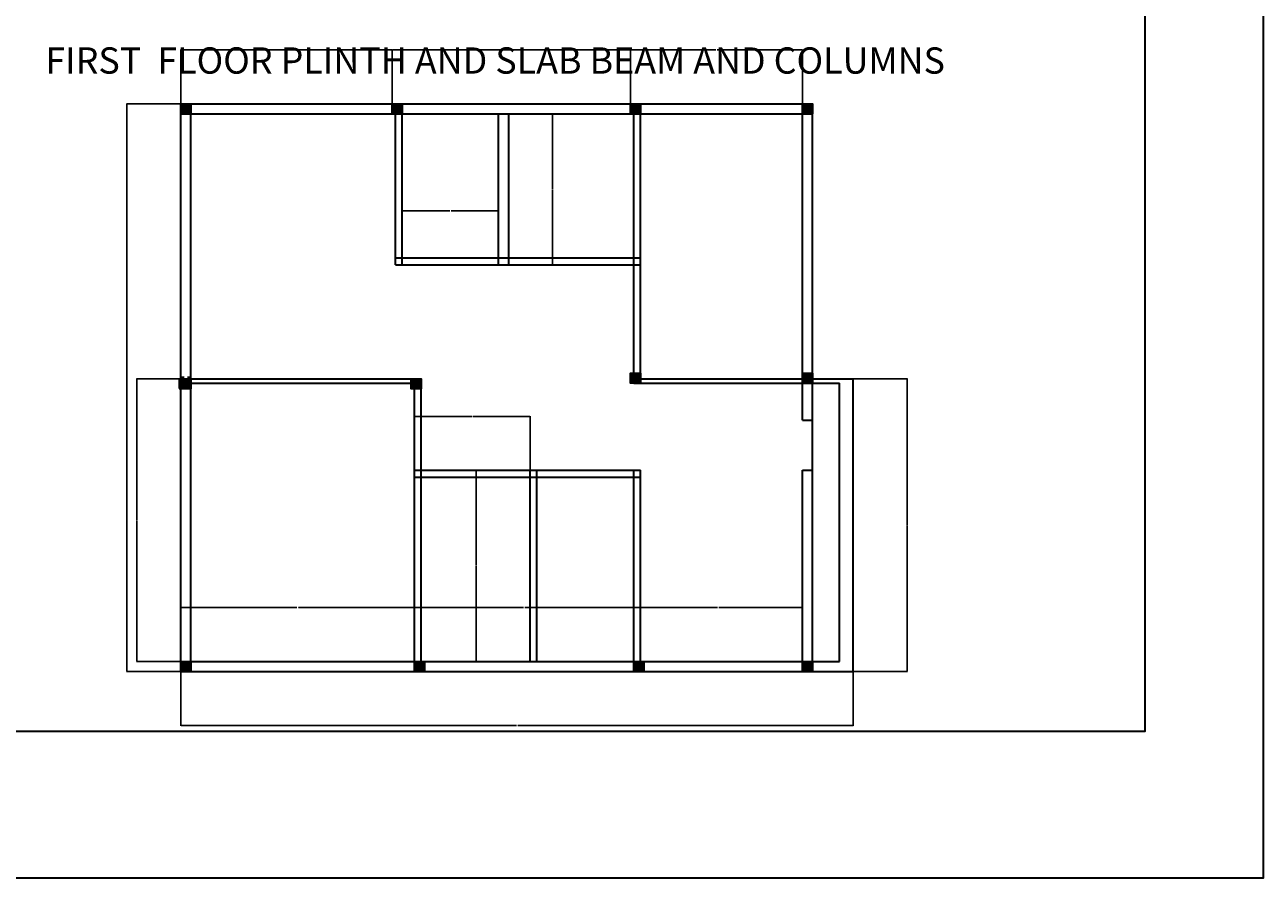
# Model space of a CAD drawing. Units: inches. Extents: x 2286 to 3750, y 1240 to 2345.
# Tile 6 of 7: x 2949 to 3750, y 1240 to 1793. Entities that reach past the tile are written whole.
import ezdxf

# ---------------------------------------------------------------- set-up
doc = ezdxf.new("R2010")
doc.units = ezdxf.units.IN
for name, color, linetype, lineweight in [('A-ANNO-DIMS', 2, 'Continuous', 18), ('A-ANNO-TEXT', 7, 'Continuous', 35), ('A-WALL', 7, 'Continuous', 35), ('S-BEAM', 7, 'Continuous', 30), ('S-COLS', 1, 'Continuous', 35)]:
    doc.layers.add(name, color=color, linetype=linetype, lineweight=lineweight)
doc.styles.get("Standard").update_dxf_attribs({"font": 'arial.ttf'})
doc.dimstyles.get("Standard").update_dxf_attribs({"dimtxt": 0.18, "dimasz": 0.18, "dimexe": 0.18, "dimexo": 0.0625, "dimgap": 0.09, "dimtad": 0, "dimtih": 1, "dimtoh": 1, "dimdec": 4, "dimzin": 0, "dimdsep": 46, "dimtxsty": 'Standard', "dimcen": 0.09, "dimadec": 0, "dimazin": 0, "dimtfac": 1, "dimtdec": 4, "dimtofl": 0, "dimtmove": 0, "dimatfit": 3, "dimfxl": 1, "dimtolj": 1, "dimtzin": 0, "dimarcsym": 0})

# ---------------------------------------------------------------- blocks, each defined once
blk = doc.blocks.new('COL-6p5-SQ')
h = blk.add_hatch(color=256)
h.dxf.hatch_style = 1
h.paths.add_polyline_path([(6.5, 0), (6.5, 6.5), (0, 6.5), (0, 0)])
blk.add_lwpolyline([(0, 6.5), (6.5, 6.5), (6.5, 0), (0, 0)], close=True)
blk = doc.blocks.new('*D20')
at = {"layer": 'A-ANNO-DIMS', "color": 0, "lineweight": -2, "transparency": 16777216}
for p, q in [((3050.31, 1563.7), (3050.31, 1564.79)), ((3050.49, 1564.61), (3052.53, 1564.61)), ((3056.63, 1564.61), (3054.6, 1564.61)), ((3056.81, 1563.7), (3056.81, 1564.79))]:
    blk.add_line(p, q, dxfattribs=at)
at = {"layer": 'A-ANNO-DIMS', "color": 0, "transparency": 16777216}
for points in [[(3050.49, 1564.64), (3050.49, 1564.58), (3050.31, 1564.61)], [(3056.63, 1564.64), (3056.63, 1564.58), (3056.81, 1564.61)]]:
    blk.add_solid(points, dxfattribs=at)
at = {"layer": 'Defpoints', "color": 0, "transparency": 16777216}
for p in [(3050.31, 1564.61), (3050.31, 1563.64), (3056.81, 1563.64)]:
    blk.add_point(p, dxfattribs=at)
at = {"layer": 'A-ANNO-DIMS', "color": 0, "transparency": 16777216, "insert": (3053.56, 1564.61), "char_height": 0.18, "attachment_point": 5}
blk.add_mtext('\\A1;COLUMN 7 TYP.', dxfattribs=at)
blk = doc.blocks.new('*D21')
at = {"layer": 'A-ANNO-DIMS', "color": 0, "lineweight": -2, "transparency": 16777216}
for p, q in [((3050.25, 1563.64), (3049.16, 1563.64)), ((3049.34, 1563.46), (3049.34, 1560.57)), ((3050.25, 1557.14), (3049.16, 1557.14)), ((3049.34, 1557.32), (3049.34, 1560.21))]:
    blk.add_line(p, q, dxfattribs=at)
at = {"layer": 'A-ANNO-DIMS', "color": 0, "transparency": 16777216}
for points in [[(3049.31, 1563.46), (3049.37, 1563.46), (3049.34, 1563.64)], [(3049.31, 1557.32), (3049.37, 1557.32), (3049.34, 1557.14)]]:
    blk.add_solid(points, dxfattribs=at)
at = {"layer": 'Defpoints', "color": 0, "transparency": 16777216}
for p in [(3050.31, 1563.64), (3049.34, 1557.14), (3050.31, 1557.14)]:
    blk.add_point(p, dxfattribs=at)
at = {"layer": 'A-ANNO-DIMS', "color": 0, "transparency": 16777216, "insert": (3049.34, 1560.39), "char_height": 0.18, "attachment_point": 5}
blk.add_mtext('\\A1;7 TYP.', dxfattribs=at)
blk = doc.blocks.new('*D109')
at = {"layer": 'A-ANNO-DIMS', "color": 0, "lineweight": -2, "transparency": 16777216}
for p, q in [((3050.31, 1374.12), (3050.31, 1339.1)), ((3485.18, 1374.12), (3485.18, 1339.1)), ((3050.49, 1339.28), (3267.35, 1339.28)), ((3485, 1339.28), (3268.14, 1339.28))]:
    blk.add_line(p, q, dxfattribs=at)
at = {"layer": 'A-ANNO-DIMS', "color": 0, "transparency": 16777216}
for points in [[(3050.49, 1339.31), (3050.49, 1339.25), (3050.31, 1339.28)], [(3485, 1339.31), (3485, 1339.25), (3485.18, 1339.28)]]:
    blk.add_solid(points, dxfattribs=at)
at = {"layer": 'Defpoints', "color": 0, "transparency": 16777216}
for p in [(3050.31, 1374.18), (3485.18, 1374.18), (3485.18, 1339.28)]:
    blk.add_point(p, dxfattribs=at)
at = {"layer": 'A-ANNO-DIMS', "color": 0, "transparency": 16777216, "insert": (3267.74, 1339.28), "char_height": 0.18, "attachment_point": 5}
blk.add_mtext('\\A1;434.9', dxfattribs=at)
blk = doc.blocks.new('*D110')
at = {"layer": 'A-ANNO-DIMS', "color": 0, "lineweight": -2, "transparency": 16777216}
for p, q in [((3050.25, 1741.52), (3015.23, 1741.52)), ((3015.41, 1741.34), (3015.41, 1558.03)), ((3015.41, 1374.36), (3015.41, 1557.67)), ((3050.24, 1374.18), (3015.23, 1374.18))]:
    blk.add_line(p, q, dxfattribs=at)
at = {"layer": 'A-ANNO-DIMS', "color": 0, "transparency": 16777216}
for points in [[(3015.38, 1741.34), (3015.44, 1741.34), (3015.41, 1741.52)], [(3015.38, 1374.36), (3015.44, 1374.36), (3015.41, 1374.18)]]:
    blk.add_solid(points, dxfattribs=at)
at = {"layer": 'Defpoints', "color": 0, "transparency": 16777216}
for p in [(3015.41, 1741.52), (3050.31, 1741.52), (3050.31, 1374.18)]:
    blk.add_point(p, dxfattribs=at)
at = {"layer": 'A-ANNO-DIMS', "color": 0, "transparency": 16777216, "insert": (3015.41, 1557.85), "char_height": 0.18, "attachment_point": 5}
blk.add_mtext('\\A1;367.34', dxfattribs=at)
blk = doc.blocks.new('*D111')
at = {"layer": 'A-ANNO-DIMS', "color": 0, "lineweight": -2, "transparency": 16777216}
for p, q in [((3050.31, 1741.58), (3050.31, 1776.61)), ((3050.49, 1776.43), (3118.19, 1776.43)), ((3186.8, 1776.43), (3119.1, 1776.43)), ((3186.98, 1741.58), (3186.98, 1776.61))]:
    blk.add_line(p, q, dxfattribs=at)
at = {"layer": 'A-ANNO-DIMS', "color": 0, "transparency": 16777216}
for points in [[(3050.49, 1776.46), (3050.49, 1776.4), (3050.31, 1776.43)], [(3186.8, 1776.46), (3186.8, 1776.4), (3186.98, 1776.43)]]:
    blk.add_solid(points, dxfattribs=at)
at = {"layer": 'Defpoints', "color": 0, "transparency": 16777216}
for p in [(3186.98, 1776.43), (3050.31, 1741.52), (3186.98, 1741.52)]:
    blk.add_point(p, dxfattribs=at)
at = {"layer": 'A-ANNO-DIMS', "color": 0, "transparency": 16777216, "insert": (3118.65, 1776.43), "char_height": 0.18, "attachment_point": 5}
blk.add_mtext('\\A1;136.67', dxfattribs=at)
blk = doc.blocks.new('*D112')
at = {"layer": 'A-ANNO-DIMS', "color": 0, "lineweight": -2, "transparency": 16777216}
for p, q in [((3186.98, 1741.58), (3186.98, 1776.61)), ((3187.16, 1776.43), (3263.54, 1776.43)), ((3340.83, 1776.43), (3264.45, 1776.43)), ((3341.01, 1741.58), (3341.01, 1776.61))]:
    blk.add_line(p, q, dxfattribs=at)
at = {"layer": 'A-ANNO-DIMS', "color": 0, "transparency": 16777216}
for points in [[(3187.16, 1776.46), (3187.16, 1776.4), (3186.98, 1776.43)], [(3340.83, 1776.46), (3340.83, 1776.4), (3341.01, 1776.43)]]:
    blk.add_solid(points, dxfattribs=at)
at = {"layer": 'Defpoints', "color": 0, "transparency": 16777216}
for p in [(3341.01, 1776.43), (3186.98, 1741.52), (3341.01, 1741.52)]:
    blk.add_point(p, dxfattribs=at)
at = {"layer": 'A-ANNO-DIMS', "color": 0, "transparency": 16777216, "insert": (3264, 1776.43), "char_height": 0.18, "attachment_point": 5}
blk.add_mtext('\\A1;154.03', dxfattribs=at)
blk = doc.blocks.new('*D113')
at = {"layer": 'A-ANNO-DIMS', "color": 0, "lineweight": -2, "transparency": 16777216}
for p, q in [((3341.01, 1741.58), (3341.01, 1776.61)), ((3341.19, 1776.43), (3396.23, 1776.43)), ((3452.19, 1776.43), (3397.14, 1776.43)), ((3452.37, 1741.58), (3452.37, 1776.61))]:
    blk.add_line(p, q, dxfattribs=at)
at = {"layer": 'A-ANNO-DIMS', "color": 0, "transparency": 16777216}
for points in [[(3341.19, 1776.46), (3341.19, 1776.4), (3341.01, 1776.43)], [(3452.19, 1776.46), (3452.19, 1776.4), (3452.37, 1776.43)]]:
    blk.add_solid(points, dxfattribs=at)
at = {"layer": 'Defpoints', "color": 0, "transparency": 16777216}
for p in [(3452.37, 1776.43), (3341.01, 1741.52), (3452.37, 1741.52)]:
    blk.add_point(p, dxfattribs=at)
at = {"layer": 'A-ANNO-DIMS', "color": 0, "transparency": 16777216, "insert": (3396.69, 1776.43), "char_height": 0.18, "attachment_point": 5}
blk.add_mtext('\\A1;111.36', dxfattribs=at)
blk = doc.blocks.new('*D114')
at = {"layer": 'A-ANNO-DIMS', "color": 0, "lineweight": -2, "transparency": 16777216}
for p, q in [((3050.31, 1380.74), (3050.31, 1415.76)), ((3050.49, 1415.58), (3125.42, 1415.58)), ((3201.26, 1415.58), (3126.33, 1415.58)), ((3201.44, 1380.74), (3201.44, 1415.76))]:
    blk.add_line(p, q, dxfattribs=at)
at = {"layer": 'A-ANNO-DIMS', "color": 0, "transparency": 16777216}
for points in [[(3050.49, 1415.61), (3050.49, 1415.55), (3050.31, 1415.58)], [(3201.26, 1415.61), (3201.26, 1415.55), (3201.44, 1415.58)]]:
    blk.add_solid(points, dxfattribs=at)
at = {"layer": 'Defpoints', "color": 0, "transparency": 16777216}
for p in [(3201.44, 1415.58), (3050.31, 1380.68), (3201.44, 1380.68)]:
    blk.add_point(p, dxfattribs=at)
at = {"layer": 'A-ANNO-DIMS', "color": 0, "transparency": 16777216, "insert": (3125.87, 1415.58), "char_height": 0.18, "attachment_point": 5}
blk.add_mtext('\\A1;151.13', dxfattribs=at)
blk = doc.blocks.new('*D115')
at = {"layer": 'A-ANNO-DIMS', "color": 0, "lineweight": -2, "transparency": 16777216}
for p, q in [((3201.44, 1380.74), (3201.44, 1415.76)), ((3201.62, 1415.58), (3271.85, 1415.58)), ((3342.99, 1415.58), (3272.76, 1415.58)), ((3343.17, 1380.74), (3343.17, 1415.76))]:
    blk.add_line(p, q, dxfattribs=at)
at = {"layer": 'A-ANNO-DIMS', "color": 0, "transparency": 16777216}
for points in [[(3201.62, 1415.61), (3201.62, 1415.55), (3201.44, 1415.58)], [(3342.99, 1415.61), (3342.99, 1415.55), (3343.17, 1415.58)]]:
    blk.add_solid(points, dxfattribs=at)
at = {"layer": 'Defpoints', "color": 0, "transparency": 16777216}
for p in [(3343.17, 1415.58), (3201.44, 1380.68), (3343.17, 1380.68)]:
    blk.add_point(p, dxfattribs=at)
at = {"layer": 'A-ANNO-DIMS', "color": 0, "transparency": 16777216, "insert": (3272.3, 1415.58), "char_height": 0.18, "attachment_point": 5}
blk.add_mtext('\\A1;141.73', dxfattribs=at)
blk = doc.blocks.new('*D116')
at = {"layer": 'A-ANNO-DIMS', "color": 0, "lineweight": -2, "transparency": 16777216}
for p, q in [((3343.17, 1380.74), (3343.17, 1415.76)), ((3343.35, 1415.58), (3397.39, 1415.58)), ((3452.19, 1415.58), (3398.15, 1415.58)), ((3452.37, 1380.74), (3452.37, 1415.76))]:
    blk.add_line(p, q, dxfattribs=at)
at = {"layer": 'A-ANNO-DIMS', "color": 0, "transparency": 16777216}
for points in [[(3343.35, 1415.61), (3343.35, 1415.55), (3343.17, 1415.58)], [(3452.19, 1415.61), (3452.19, 1415.55), (3452.37, 1415.58)]]:
    blk.add_solid(points, dxfattribs=at)
at = {"layer": 'Defpoints', "color": 0, "transparency": 16777216}
for p in [(3452.37, 1415.58), (3343.17, 1380.68), (3452.37, 1380.68)]:
    blk.add_point(p, dxfattribs=at)
at = {"layer": 'A-ANNO-DIMS', "color": 0, "transparency": 16777216, "insert": (3397.77, 1415.58), "char_height": 0.18, "attachment_point": 5}
blk.add_mtext('\\A1;109.2', dxfattribs=at)
blk = doc.blocks.new('*D117')
at = {"layer": 'A-ANNO-DIMS', "color": 0, "lineweight": -2, "transparency": 16777216}
for p, q in [((3056.75, 1563.64), (3021.73, 1563.64)), ((3021.91, 1563.46), (3021.91, 1472.34)), ((3021.91, 1380.86), (3021.91, 1471.98)), ((3056.74, 1380.68), (3021.73, 1380.68))]:
    blk.add_line(p, q, dxfattribs=at)
at = {"layer": 'A-ANNO-DIMS', "color": 0, "transparency": 16777216}
for points in [[(3021.88, 1563.46), (3021.94, 1563.46), (3021.91, 1563.64)], [(3021.88, 1380.86), (3021.94, 1380.86), (3021.91, 1380.68)]]:
    blk.add_solid(points, dxfattribs=at)
at = {"layer": 'Defpoints', "color": 0, "transparency": 16777216}
for p in [(3021.91, 1563.64), (3056.81, 1563.64), (3056.81, 1380.68)]:
    blk.add_point(p, dxfattribs=at)
at = {"layer": 'A-ANNO-DIMS', "color": 0, "transparency": 16777216, "insert": (3021.91, 1472.16), "char_height": 0.18, "attachment_point": 5}
blk.add_mtext('\\A1;182.96', dxfattribs=at)
blk = doc.blocks.new('*D118')
at = {"layer": 'A-ANNO-DIMS', "color": 0, "lineweight": -2, "transparency": 16777216}
for p, q in [((3485.24, 1563.64), (3520.26, 1563.64)), ((3520.08, 1563.46), (3520.08, 1469.09)), ((3520.08, 1374.36), (3520.08, 1468.73)), ((3485.24, 1374.18), (3520.26, 1374.18))]:
    blk.add_line(p, q, dxfattribs=at)
at = {"layer": 'A-ANNO-DIMS', "color": 0, "transparency": 16777216}
for points in [[(3520.05, 1563.46), (3520.11, 1563.46), (3520.08, 1563.64)], [(3520.05, 1374.36), (3520.11, 1374.36), (3520.08, 1374.18)]]:
    blk.add_solid(points, dxfattribs=at)
at = {"layer": 'Defpoints', "color": 0, "transparency": 16777216}
for p in [(3485.18, 1563.64), (3520.08, 1563.64), (3485.18, 1374.18)]:
    blk.add_point(p, dxfattribs=at)
at = {"layer": 'A-ANNO-DIMS', "color": 0, "transparency": 16777216, "insert": (3520.08, 1468.91), "char_height": 0.18, "attachment_point": 5}
blk.add_mtext('\\A1;189.46', dxfattribs=at)
blk = doc.blocks.new('*D119')
at = {"layer": 'A-ANNO-DIMS', "color": 0, "lineweight": -2, "transparency": 16777216}
for p, q in [((3193.48, 1637.46), (3193.48, 1672.48)), ((3193.66, 1672.3), (3224.27, 1672.3)), ((3255.66, 1672.3), (3225.06, 1672.3)), ((3255.84, 1637.46), (3255.84, 1672.48))]:
    blk.add_line(p, q, dxfattribs=at)
at = {"layer": 'A-ANNO-DIMS', "color": 0, "transparency": 16777216}
for points in [[(3193.66, 1672.33), (3193.66, 1672.27), (3193.48, 1672.3)], [(3255.66, 1672.33), (3255.66, 1672.27), (3255.84, 1672.3)]]:
    blk.add_solid(points, dxfattribs=at)
at = {"layer": 'Defpoints', "color": 0, "transparency": 16777216}
for p in [(3255.84, 1672.3), (3193.48, 1637.4), (3255.84, 1637.4)]:
    blk.add_point(p, dxfattribs=at)
at = {"layer": 'A-ANNO-DIMS', "color": 0, "transparency": 16777216, "insert": (3224.66, 1672.3), "char_height": 0.18, "attachment_point": 5}
blk.add_mtext('\\A1;62.36', dxfattribs=at)
blk = doc.blocks.new('*D120')
at = {"layer": 'A-ANNO-DIMS', "color": 0, "lineweight": -2, "transparency": 16777216}
for p, q in [((3255.9, 1735.02), (3290.92, 1735.02)), ((3290.74, 1734.84), (3290.74, 1686.39)), ((3290.74, 1637.58), (3290.74, 1686.03)), ((3255.9, 1637.4), (3290.92, 1637.4))]:
    blk.add_line(p, q, dxfattribs=at)
at = {"layer": 'A-ANNO-DIMS', "color": 0, "transparency": 16777216}
for points in [[(3290.71, 1734.84), (3290.77, 1734.84), (3290.74, 1735.02)], [(3290.71, 1637.58), (3290.77, 1637.58), (3290.74, 1637.4)]]:
    blk.add_solid(points, dxfattribs=at)
at = {"layer": 'Defpoints', "color": 0, "transparency": 16777216}
for p in [(3255.84, 1735.02), (3255.84, 1637.4), (3290.74, 1637.4)]:
    blk.add_point(p, dxfattribs=at)
at = {"layer": 'A-ANNO-DIMS', "color": 0, "transparency": 16777216, "insert": (3290.74, 1686.21), "char_height": 0.18, "attachment_point": 5}
blk.add_mtext('\\A1;97.62', dxfattribs=at)
blk = doc.blocks.new('*D121')
at = {"layer": 'A-ANNO-DIMS', "color": 0, "lineweight": -2, "transparency": 16777216}
for p, q in [((3201.44, 1504.4), (3201.44, 1539.42)), ((3201.62, 1539.24), (3238.44, 1539.24)), ((3276.05, 1539.24), (3239.23, 1539.24)), ((3276.23, 1504.4), (3276.23, 1539.42))]:
    blk.add_line(p, q, dxfattribs=at)
at = {"layer": 'A-ANNO-DIMS', "color": 0, "transparency": 16777216}
for points in [[(3201.62, 1539.27), (3201.62, 1539.21), (3201.44, 1539.24)], [(3276.05, 1539.27), (3276.05, 1539.21), (3276.23, 1539.24)]]:
    blk.add_solid(points, dxfattribs=at)
at = {"layer": 'Defpoints', "color": 0, "transparency": 16777216}
for p in [(3276.23, 1539.24), (3201.44, 1504.34), (3276.23, 1504.34)]:
    blk.add_point(p, dxfattribs=at)
at = {"layer": 'A-ANNO-DIMS', "color": 0, "transparency": 16777216, "insert": (3238.83, 1539.24), "char_height": 0.18, "attachment_point": 5}
blk.add_mtext('\\A1;74.79', dxfattribs=at)
blk = doc.blocks.new('*D122')
at = {"layer": 'A-ANNO-DIMS', "color": 0, "lineweight": -2, "transparency": 16777216}
for p, q in [((3276.16, 1504.34), (3241.15, 1504.34)), ((3241.33, 1504.16), (3241.33, 1442.7)), ((3241.33, 1380.87), (3241.33, 1442.33)), ((3276.16, 1380.69), (3241.15, 1380.69))]:
    blk.add_line(p, q, dxfattribs=at)
at = {"layer": 'A-ANNO-DIMS', "color": 0, "transparency": 16777216}
for points in [[(3241.3, 1504.16), (3241.36, 1504.16), (3241.33, 1504.34)], [(3241.3, 1380.87), (3241.36, 1380.87), (3241.33, 1380.69)]]:
    blk.add_solid(points, dxfattribs=at)
at = {"layer": 'Defpoints', "color": 0, "transparency": 16777216}
for p in [(3241.33, 1504.34), (3276.23, 1504.34), (3276.23, 1380.69)]:
    blk.add_point(p, dxfattribs=at)
at = {"layer": 'A-ANNO-DIMS', "color": 0, "transparency": 16777216, "insert": (3241.33, 1442.52), "char_height": 0.18, "attachment_point": 5}
blk.add_mtext('\\A1;123.65', dxfattribs=at)

msp = doc.modelspace()

# ---------------------------------------------------------------- linework, layer by layer
at = {"layer": 'A-WALL'}
for points in [[(2286.2079, 2344.8717), (3750.2574, 2344.8717), (3750.2574, 1240.4105), (2286.2079, 1240.4105)], [(2354.794, 2286.8809), (3673.7575, 2286.8809), (3673.7575, 1335.3046), (2354.794, 1335.3046)]]:
    msp.add_lwpolyline(points, close=True, dxfattribs=at)
at = {"layer": 'S-BEAM'}
for p, q in [((3050.3051, 1741.5266), (3458.8692, 1741.5266)), ((3050.3051, 1374.1804), (3050.3051, 1741.5266)), ((3056.8132, 1380.6885), (3056.8132, 1741.5266)), ((3189.1446, 1637.397), (3189.1446, 1741.5266)), ((3193.4833, 1637.397), (3193.4833, 1741.5266)), ((3343.1697, 1560.746), (3343.1697, 1741.5266)), ((3347.5084, 1560.746), (3347.5084, 1741.5266)), ((3452.3611, 1536.746), (3452.3611, 1741.5266)), ((3458.8692, 1374.1804), (3458.8692, 1741.5266)), ((3050.3051, 1735.0185), (3458.8692, 1735.0185)), ((3056.8132, 1674.2762), (3056.8132, 1735.0185)), ((3255.8397, 1637.397), (3255.8397, 1735.0185)), ((3262.3478, 1637.397), (3262.3478, 1735.0185)), ((3189.1446, 1641.7357), (3347.5084, 1641.7357)), ((3189.1446, 1637.397), (3347.5084, 1637.397)), ((3050.3051, 1563.6385), (3205.7764, 1563.6385)), ((3201.4377, 1374.1804), (3201.4377, 1563.6385)), ((3205.7764, 1380.6885), (3205.7764, 1563.6385)), ((3343.1697, 1563.6385), (3485.18, 1563.6385)), ((3485.18, 1374.1804), (3485.18, 1563.6385)), ((3050.3051, 1560.746), (3205.7764, 1560.746)), ((3343.1697, 1560.746), (3476.18, 1560.746)), ((3476.18, 1380.6885), (3476.18, 1560.746)), ((3452.3611, 1536.746), (3458.8692, 1536.746)), ((3201.4377, 1504.3424), (3205.7764, 1504.3424)), ((3201.4377, 1500.0037), (3205.7764, 1500.0037)), ((3205.7764, 1504.3424), (3347.5084, 1504.3424)), ((3205.7764, 1500.0037), (3347.5084, 1500.0037)), ((3276.227, 1380.6885), (3276.227, 1504.3424)), ((3280.5657, 1380.6885), (3280.5657, 1504.3424)), ((3343.1697, 1374.1804), (3343.1697, 1504.3424)), ((3347.5084, 1374.1804), (3347.5084, 1504.3424)), ((3452.3611, 1504.3424), (3458.8692, 1504.3424)), ((3452.3611, 1380.6885), (3452.3611, 1504.3424)), ((3050.3051, 1380.6885), (3476.18, 1380.6885)), ((3050.3051, 1374.1804), (3485.18, 1374.1804))]:
    msp.add_line(p, q, dxfattribs=at)

# ---------------------------------------------------------------- block references
at = {"layer": 'S-COLS', "rotation": 180}
for p in [(3056.8132, 1741.5185), (3193.4833, 1741.5185), (3347.5084, 1741.5185), (3056.8132, 1563.6385), (3205.7764, 1563.6385), (3347.5084, 1567.246), (3458.8692, 1567.246), (3056.8051, 1380.6804), (3207.9377, 1380.6804), (3349.6697, 1380.6804), (3458.8692, 1380.6804)]:
    msp.add_blockref('COL-6p5-SQ', p, dxfattribs=at)
at = {"layer": 'S-COLS'}
msp.add_blockref('COL-6p5-SQ', (3452.3692, 1735.0185), dxfattribs=at)

# ---------------------------------------------------------------- texts
at = {"layer": 'A-ANNO-TEXT'}
msp.add_text('FIRST  FLOOR PLINTH AND SLAB BEAM AND COLUMNS', height=17, dxfattribs=at).set_placement((2962.6875, 1761.0035))

# ---------------------------------------------------------------- dimensions: what is measured, and where the dimension line sits
at = {"layer": 'A-ANNO-DIMS'}
for base, p1, p2, override, picture, middle in [((3186.9833, 1776.4266), (3050.3132, 1741.5185), (3186.9833, 1741.5185), {"dimdec": 2, "dimlfac": 1, "dimrnd": 0, "dimzin": 0, "dimdsep": 46, "dimlunit": 2}, '*D111', (3118.6482, 1776.4266)), ((3341.0084, 1776.4266), (3186.9833, 1741.5185), (3341.0084, 1741.5185), {"dimdec": 2, "dimlfac": 1, "dimrnd": 0, "dimzin": 0, "dimdsep": 46, "dimlunit": 2}, '*D112', (3263.9959, 1776.4266)), ((3452.3692, 1776.4266), (3341.0084, 1741.5185), (3452.3692, 1741.5185), {"dimdec": 2, "dimlfac": 1, "dimrnd": 0, "dimzin": 0, "dimdsep": 46, "dimlunit": 2}, '*D113', (3396.6888, 1776.4266)), ((3255.8397, 1672.297), (3193.4833, 1637.397), (3255.8397, 1637.397), {"dimdec": 2, "dimlfac": 1, "dimrnd": 0, "dimzin": 0, "dimdsep": 46, "dimlunit": 2}, '*D119', (3224.6615, 1672.297)), ((3276.227, 1539.2424), (3201.4377, 1504.3424), (3276.227, 1504.3424), {"dimdec": 2, "dimlfac": 1, "dimrnd": 0, "dimzin": 0, "dimdsep": 46, "dimlunit": 2}, '*D121', (3238.8323, 1539.2424)), ((3201.4377, 1415.5804), (3050.3051, 1380.6804), (3201.4377, 1380.6804), {"dimdec": 2, "dimlfac": 1, "dimrnd": 0, "dimzin": 0, "dimdsep": 46, "dimlunit": 2}, '*D114', (3125.8714, 1415.5804)), ((3343.1697, 1415.5804), (3201.4377, 1380.6804), (3343.1697, 1380.6804), {"dimdec": 2, "dimlfac": 1, "dimrnd": 0, "dimzin": 0, "dimdsep": 46, "dimlunit": 2}, '*D115', (3272.3037, 1415.5804)), ((3452.3692, 1415.5804), (3343.1697, 1380.6804), (3452.3692, 1380.6804), {"dimdec": 1, "dimlfac": 1, "dimrnd": 0, "dimzin": 0, "dimdsep": 46, "dimlunit": 2}, '*D116', (3397.7695, 1415.5804)), ((3485.18, 1339.2804), (3050.3051, 1374.1804), (3485.18, 1374.1804), {"dimdec": 1, "dimlfac": 1, "dimrnd": 0, "dimzin": 0, "dimdsep": 46, "dimlunit": 2}, '*D109', (3267.7425, 1339.2804))]:
    dim = msp.add_linear_dim(base=base, p1=p1, p2=p2, dimstyle='Standard', override=override, dxfattribs=at)
    dim.commit()
    dim.dimension.update_dxf_attribs({"geometry": picture, "text_midpoint": middle})
for base, p1, p2, angle, picture, middle in [((3015.4051, 1741.5185), (3050.3051, 1374.1804), (3050.3132, 1741.5185), 90, '*D110', (3015.4051, 1557.8494)), ((3290.7397, 1637.397), (3255.8397, 1735.0185), (3255.8397, 1637.397), 270, '*D120', (3290.7397, 1686.2077)), ((3021.9132, 1563.64), (3056.8051, 1380.6804), (3056.8132, 1563.6385), 89.9974628, '*D117', (3021.9091, 1472.161)), ((3520.08, 1563.6385), (3485.18, 1374.1804), (3485.18, 1563.6385), 90, '*D118', (3520.08, 1468.9094)), ((3241.327, 1504.3424), (3276.227, 1380.6885), (3276.227, 1504.3424), 90, '*D122', (3241.327, 1442.5155))]:
    dim = msp.add_linear_dim(base=base, p1=p1, p2=p2, angle=angle, dimstyle='Standard', override={"dimdec": 2, "dimlfac": 1, "dimrnd": 0, "dimzin": 0, "dimdsep": 46, "dimlunit": 2}, dxfattribs=at)
    dim.commit()
    dim.dimension.update_dxf_attribs({"geometry": picture, "text_midpoint": middle})
for base, p1, p2, angle, text, picture, middle in [((3049.3381803596, 1557.1384684059), (3050.3131803596, 1563.6384684059), (3050.3131803596, 1557.1384684059), 270, '<> TYP.', '*D21', (3049.3381803596, 1560.3884684059)), ((3050.3131803596, 1564.6134684059), (3056.8131803596, 1563.6384684059), (3050.3131803596, 1563.6384684059), 180, 'COLUMN <> TYP.', '*D20', (3053.5631803596, 1564.6134684059))]:
    dim = msp.add_linear_dim(base=base, p1=p1, p2=p2, angle=angle, text=text, dimstyle='Standard', override={"dimdec": 0, "dimlfac": 1, "dimrnd": 0, "dimzin": 0, "dimdsep": 46, "dimlunit": 2}, dxfattribs=at)
    dim.commit()
    dim.dimension.update_dxf_attribs({"geometry": picture, "text_midpoint": middle})

doc.saveas('drawing.dxf')
